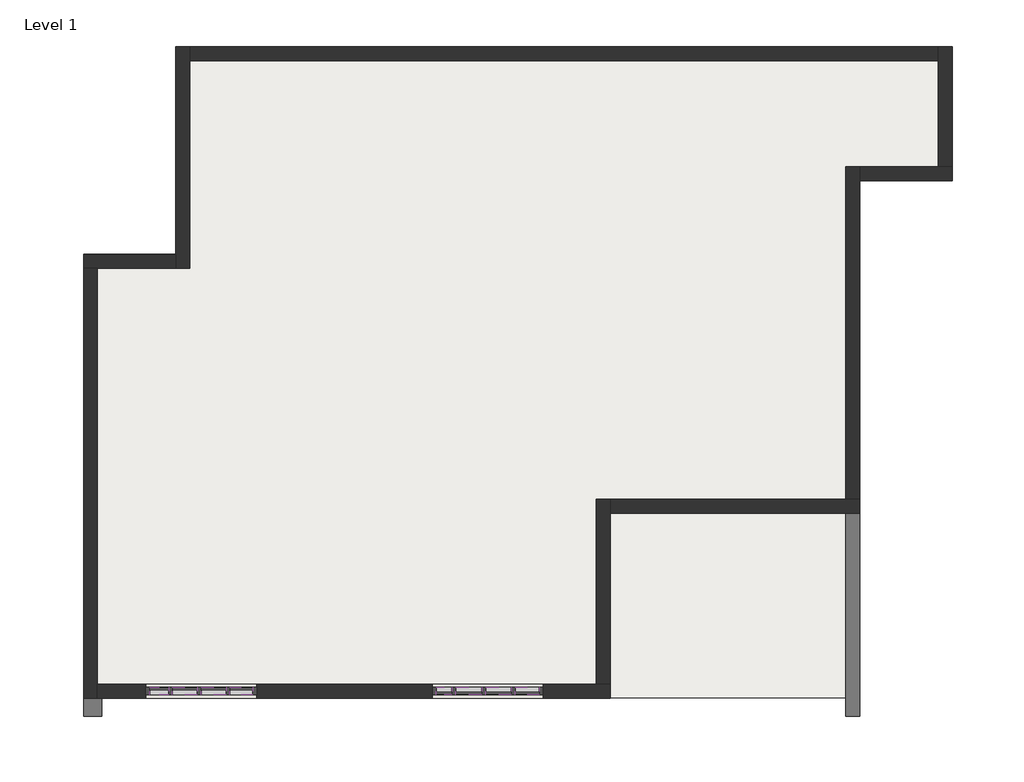
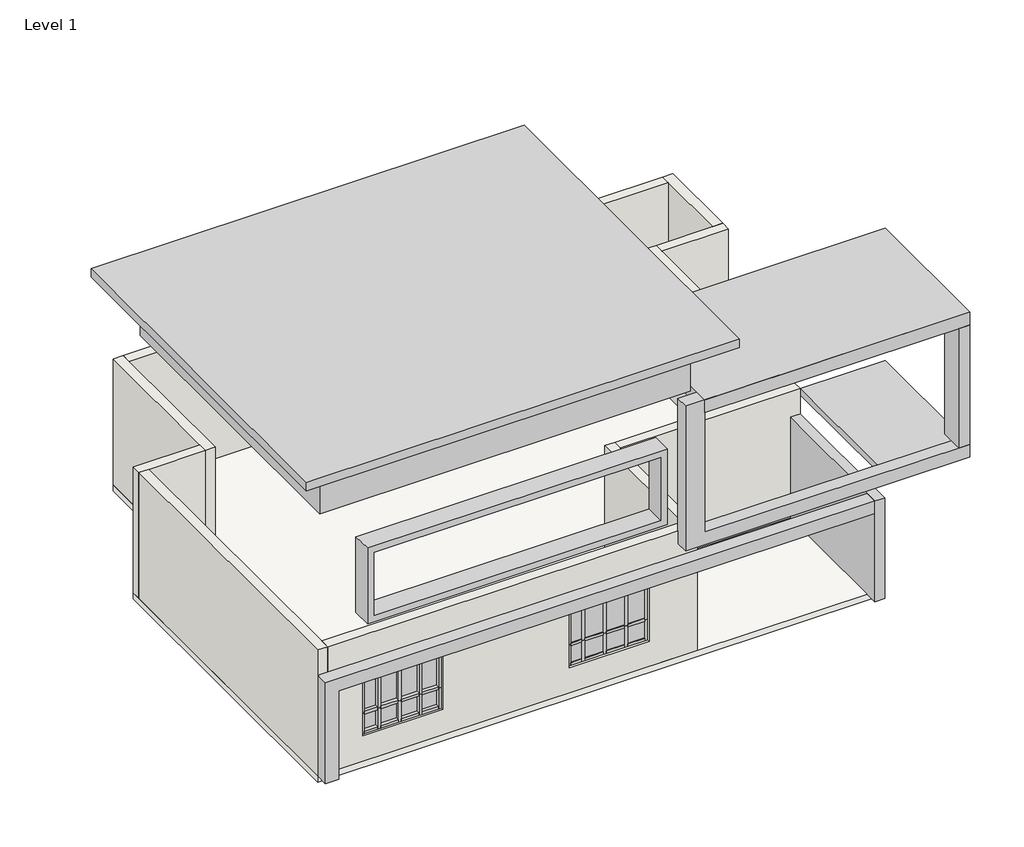
# One storey: 44 members, 16 plates, 10 walls, 1 proxy, 1 slab.
"""IFC4 building model written with IfcOpenShell, lengths in millimetres."""

from ifc_helpers import new_model, si_unit, frame, origin, origin_with_axes, place, context, project, spatial, polyline, outline, extrude, faceted_brep, transform, mapped, element, save
from components import generic_models_1_generic_models_1_da173db9, member_35330a42, member_5ad95953, member_90750a43, member_9850ab14, member_34d525fb, member_e756d367, member_8b1256c5, member_f92b8aa2, member_8e09d03a, member_7fd687a9, member_4adcbd6e, member_1c9dfce7, member_5ca2cede, member_be2dbdeb, member_cf238b44, member_39486dda, system_panel_glazed_bc497e33, system_panel_glazed_3f4378e1, system_panel_glazed_eeed78fb, system_panel_glazed_60bba13d, system_panel_glazed_ad989134, system_panel_glazed_d518dbe9, system_panel_glazed_4258910c, system_panel_glazed_d839e02d, system_panel_glazed_c56bea94, system_panel_glazed_323f7165, system_panel_glazed_9bb7629d, system_panel_glazed_ece2a562

model = new_model("IFC4")

# Units and contexts
model_context = context("Model", 3, world=origin())
ifc_project = project(units=[si_unit("LENGTHUNIT", "METRE", prefix="MILLI")], contexts=[model_context])

# Site, building, storey
site = spatial("IfcSite", under=ifc_project)
building = spatial("IfcBuilding", under=site)
storey = spatial("IfcBuildingStorey", under=building, Name="Level 1", Elevation=0.0)

# Proxy
placement = place(None, origin())
generic_models_1_generic_models_1_shape = generic_models_1_generic_models_1_da173db9(model_context)
element("IfcBuildingElementProxy", 1, Name="Generic Models 1 : Generic Models 1", ObjectType="Generic Models 1 : Generic Models 1", at=placement, inside=storey, context=model_context, shape_type="MappedRepresentation", body=[
    mapped(generic_models_1_generic_models_1_shape, transform((0.0, 0.0, 0.0), x_axis=(1.0, 0.0, 0.0), y_axis=(0.0, 1.0, 0.0), z_axis=(0.0, 0.0, 1.0))),
])

# Members
member_shape = member_35330a42(model_context)
element("IfcMember", 2, ObjectType="Rectangular Mullion : 2.5\" x 5\" rectangular", at=placement, inside=storey, context=model_context, shape_type="MappedRepresentation", body=[
    mapped(member_shape, transform((-4793.1680265, 1641.9286055, 2133.6), x_axis=(0.0, 0.0, 1.0), y_axis=(0.0, -1.0, 0.0), z_axis=(1.0, 0.0, 0.0))),
])
member_2_shape = member_5ad95953(model_context)
element("IfcMember", 3, ObjectType="Rectangular Mullion : 2.5\" x 5\" rectangular", at=placement, inside=storey, context=model_context, shape_type="MappedRepresentation", body=[
    mapped(member_2_shape, transform((-6494.9680265, 1641.9286055, 609.6), x_axis=(0.0, 0.0, -1.0), y_axis=(0.0, -1.0, 0.0), z_axis=(-1.0, 0.0, 0.0))),
])
member_3_shape = member_90750a43(model_context)
element("IfcMember", 4, ObjectType="Rectangular Mullion : 2.5\" x 5\" rectangular", at=placement, inside=storey, context=model_context, shape_type="MappedRepresentation", body=[
    mapped(member_3_shape, transform((-6152.0680265, 1641.9286055, 609.6), x_axis=(1.0, 0.0, 0.0), y_axis=(0.0, -1.0, 0.0), z_axis=(0.0, 0.0, -1.0))),
])
element("IfcMember", 5, ObjectType="Rectangular Mullion : 2.5\" x 5\" rectangular", at=placement, inside=storey, context=model_context, shape_type="MappedRepresentation", body=[
    mapped(member_3_shape, transform((-5677.9346932, 1641.9286055, 609.6), x_axis=(1.0, 0.0, 0.0), y_axis=(0.0, -1.0, 0.0), z_axis=(0.0, 0.0, -1.0))),
])
element("IfcMember", 6, ObjectType="Rectangular Mullion : 2.5\" x 5\" rectangular", at=placement, inside=storey, context=model_context, shape_type="MappedRepresentation", body=[
    mapped(member_3_shape, transform((-5203.8013599, 1641.9286055, 609.6), x_axis=(1.0, 0.0, 0.0), y_axis=(0.0, -1.0, 0.0), z_axis=(0.0, 0.0, -1.0))),
])
element("IfcMember", 7, ObjectType="Rectangular Mullion : 2.5\" x 5\" rectangular", at=placement, inside=storey, context=model_context, shape_type="MappedRepresentation", body=[
    mapped(member_3_shape, transform((-1478.4680265, 1641.9286055, 609.6), x_axis=(-1.0, 0.0, 0.0), y_axis=(0.0, 1.0, 0.0), z_axis=(0.0, 0.0, -1.0))),
])
element("IfcMember", 8, ObjectType="Rectangular Mullion : 2.5\" x 5\" rectangular", at=placement, inside=storey, context=model_context, shape_type="MappedRepresentation", body=[
    mapped(member_3_shape, transform((-987.4013599, 1641.9286055, 609.6), x_axis=(-1.0, 0.0, 0.0), y_axis=(0.0, 1.0, 0.0), z_axis=(0.0, 0.0, -1.0))),
])
element("IfcMember", 9, ObjectType="Rectangular Mullion : 2.5\" x 5\" rectangular", at=placement, inside=storey, context=model_context, shape_type="MappedRepresentation", body=[
    mapped(member_3_shape, transform((-496.3346932, 1641.9286055, 609.6), x_axis=(-1.0, 0.0, 0.0), y_axis=(0.0, 1.0, 0.0), z_axis=(0.0, 0.0, -1.0))),
])
member_4_shape = member_9850ab14(model_context)
element("IfcMember", 10, ObjectType="Rectangular Mullion : 2.5\" x 5\" rectangular", at=placement, inside=storey, context=model_context, shape_type="MappedRepresentation", body=[
    mapped(member_4_shape, transform((-6183.8180265, 1641.9286055, 1117.6), x_axis=(0.0, 0.0, 1.0), y_axis=(0.0, -1.0, 0.0), z_axis=(1.0, 0.0, 0.0))),
])
member_5_shape = member_34d525fb(model_context)
element("IfcMember", 11, ObjectType="Rectangular Mullion : 2.5\" x 5\" rectangular", at=placement, inside=storey, context=model_context, shape_type="MappedRepresentation", body=[
    mapped(member_5_shape, transform((-5709.6846932, 1641.9286055, 1117.6), x_axis=(0.0, 0.0, 1.0), y_axis=(0.0, -1.0, 0.0), z_axis=(1.0, 0.0, 0.0))),
])
element("IfcMember", 12, ObjectType="Rectangular Mullion : 2.5\" x 5\" rectangular", at=placement, inside=storey, context=model_context, shape_type="MappedRepresentation", body=[
    mapped(member_5_shape, transform((-5235.5513599, 1641.9286055, 1117.6), x_axis=(0.0, 0.0, 1.0), y_axis=(0.0, -1.0, 0.0), z_axis=(1.0, 0.0, 0.0))),
])
member_6_shape = member_e756d367(model_context)
element("IfcMember", 13, ObjectType="Rectangular Mullion : 2.5\" x 5\" rectangular", at=placement, inside=storey, context=model_context, shape_type="MappedRepresentation", body=[
    mapped(member_6_shape, transform((-4793.1680265, 1641.9286055, 1117.6), x_axis=(0.0, 0.0, 1.0), y_axis=(0.0, -1.0, 0.0), z_axis=(1.0, 0.0, 0.0))),
])
member_7_shape = member_8b1256c5(model_context)
element("IfcMember", 14, ObjectType="Rectangular Mullion : 2.5\" x 5\" rectangular", at=placement, inside=storey, context=model_context, shape_type="MappedRepresentation", body=[
    mapped(member_7_shape, transform((-6120.3180265, 1641.9286055, 609.6), x_axis=(0.0, 0.0, -1.0), y_axis=(0.0, -1.0, 0.0), z_axis=(-1.0, 0.0, 0.0))),
])
element("IfcMember", 15, ObjectType="Rectangular Mullion : 2.5\" x 5\" rectangular", at=placement, inside=storey, context=model_context, shape_type="MappedRepresentation", body=[
    mapped(member_7_shape, transform((-5646.1846932, 1641.9286055, 609.6), x_axis=(0.0, 0.0, -1.0), y_axis=(0.0, -1.0, 0.0), z_axis=(-1.0, 0.0, 0.0))),
])
element("IfcMember", 16, ObjectType="Rectangular Mullion : 2.5\" x 5\" rectangular", at=placement, inside=storey, context=model_context, shape_type="MappedRepresentation", body=[
    mapped(member_shape, transform((-5172.0513599, 1641.9286055, 609.6), x_axis=(0.0, 0.0, -1.0), y_axis=(0.0, -1.0, 0.0), z_axis=(-1.0, 0.0, 0.0))),
])
element("IfcMember", 17, ObjectType="Rectangular Mullion : 2.5\" x 5\" rectangular", at=placement, inside=storey, context=model_context, shape_type="MappedRepresentation", body=[
    mapped(member_2_shape, transform((-6183.8180265, 1641.9286055, 2133.6), x_axis=(0.0, 0.0, 1.0), y_axis=(0.0, -1.0, 0.0), z_axis=(1.0, 0.0, 0.0))),
])
element("IfcMember", 18, ObjectType="Rectangular Mullion : 2.5\" x 5\" rectangular", at=placement, inside=storey, context=model_context, shape_type="MappedRepresentation", body=[
    mapped(member_7_shape, transform((-5709.6846932, 1641.9286055, 2133.6), x_axis=(0.0, 0.0, 1.0), y_axis=(0.0, -1.0, 0.0), z_axis=(1.0, 0.0, 0.0))),
])
element("IfcMember", 19, ObjectType="Rectangular Mullion : 2.5\" x 5\" rectangular", at=placement, inside=storey, context=model_context, shape_type="MappedRepresentation", body=[
    mapped(member_7_shape, transform((-5235.5513599, 1641.9286055, 2133.6), x_axis=(0.0, 0.0, 1.0), y_axis=(0.0, -1.0, 0.0), z_axis=(1.0, 0.0, 0.0))),
])
member_8_shape = member_f92b8aa2(model_context)
element("IfcMember", 20, ObjectType="Rectangular Mullion : 2.5\" x 5\" rectangular", at=placement, inside=storey, context=model_context, shape_type="MappedRepresentation", body=[
    mapped(member_8_shape, transform((-6152.0680265, 1641.9286055, 1117.6), x_axis=(1.0, 0.0, 0.0), y_axis=(0.0, -1.0, 0.0), z_axis=(0.0, 0.0, -1.0))),
])
element("IfcMember", 21, ObjectType="Rectangular Mullion : 2.5\" x 5\" rectangular", at=placement, inside=storey, context=model_context, shape_type="MappedRepresentation", body=[
    mapped(member_8_shape, transform((-5677.9346932, 1641.9286055, 1117.6), x_axis=(1.0, 0.0, 0.0), y_axis=(0.0, -1.0, 0.0), z_axis=(0.0, 0.0, -1.0))),
])
element("IfcMember", 22, ObjectType="Rectangular Mullion : 2.5\" x 5\" rectangular", at=placement, inside=storey, context=model_context, shape_type="MappedRepresentation", body=[
    mapped(member_8_shape, transform((-5203.8013599, 1641.9286055, 1117.6), x_axis=(1.0, 0.0, 0.0), y_axis=(0.0, -1.0, 0.0), z_axis=(0.0, 0.0, -1.0))),
])
element("IfcMember", 23, ObjectType="Rectangular Mullion : 2.5\" x 5\" rectangular", at=placement, inside=storey, context=model_context, shape_type="MappedRepresentation", body=[
    mapped(member_8_shape, transform((-1478.4680265, 1641.9286055, 1117.6), x_axis=(-1.0, 0.0, 0.0), y_axis=(0.0, 1.0, 0.0), z_axis=(0.0, 0.0, -1.0))),
])
element("IfcMember", 24, ObjectType="Rectangular Mullion : 2.5\" x 5\" rectangular", at=placement, inside=storey, context=model_context, shape_type="MappedRepresentation", body=[
    mapped(member_8_shape, transform((-987.4013599, 1641.9286055, 1117.6), x_axis=(-1.0, 0.0, 0.0), y_axis=(0.0, 1.0, 0.0), z_axis=(0.0, 0.0, -1.0))),
])
element("IfcMember", 25, ObjectType="Rectangular Mullion : 2.5\" x 5\" rectangular", at=placement, inside=storey, context=model_context, shape_type="MappedRepresentation", body=[
    mapped(member_8_shape, transform((-496.3346932, 1641.9286055, 1117.6), x_axis=(-1.0, 0.0, 0.0), y_axis=(0.0, 1.0, 0.0), z_axis=(0.0, 0.0, -1.0))),
])
member_9_shape = member_8e09d03a(model_context)
element("IfcMember", 26, ObjectType="Rectangular Mullion : 2.5\" x 5\" rectangular", at=placement, inside=storey, context=model_context, shape_type="MappedRepresentation", body=[
    mapped(member_9_shape, transform((-6558.4680265, 1641.9286055, 2133.6), x_axis=(-1.0, 0.0, 0.0), y_axis=(0.0, -1.0, 0.0), z_axis=(0.0, 0.0, 1.0))),
])
element("IfcMember", 27, ObjectType="Rectangular Mullion : 2.5\" x 5\" rectangular", at=placement, inside=storey, context=model_context, shape_type="MappedRepresentation", body=[
    mapped(member_9_shape, transform((-5.2680265, 1641.9286055, 2133.6), x_axis=(1.0, 0.0, 0.0), y_axis=(0.0, 1.0, 0.0), z_axis=(0.0, 0.0, 1.0))),
])
member_10_shape = member_7fd687a9(model_context)
element("IfcMember", 28, ObjectType="Rectangular Mullion : 2.5\" x 5\" rectangular", at=placement, inside=storey, context=model_context, shape_type="MappedRepresentation", body=[
    mapped(member_10_shape, transform((-4729.6680265, 1641.9286055, 609.6), x_axis=(1.0, 0.0, 0.0), y_axis=(0.0, -1.0, 0.0), z_axis=(0.0, 0.0, -1.0))),
])
element("IfcMember", 29, ObjectType="Rectangular Mullion : 2.5\" x 5\" rectangular", at=placement, inside=storey, context=model_context, shape_type="MappedRepresentation", body=[
    mapped(member_10_shape, transform((-1834.0680265, 1641.9286055, 609.6), x_axis=(-1.0, 0.0, 0.0), y_axis=(0.0, 1.0, 0.0), z_axis=(0.0, 0.0, -1.0))),
])
element("IfcMember", 30, ObjectType="Rectangular Mullion : 2.5\" x 5\" rectangular", at=placement, inside=storey, context=model_context, shape_type="MappedRepresentation", body=[
    mapped(member_9_shape, transform((-4729.6680265, 1641.9286055, 1117.6), x_axis=(1.0, 0.0, 0.0), y_axis=(0.0, -1.0, 0.0), z_axis=(0.0, 0.0, -1.0))),
])
element("IfcMember", 31, ObjectType="Rectangular Mullion : 2.5\" x 5\" rectangular", at=placement, inside=storey, context=model_context, shape_type="MappedRepresentation", body=[
    mapped(member_9_shape, transform((-1834.0680265, 1641.9286055, 1117.6), x_axis=(-1.0, 0.0, 0.0), y_axis=(0.0, 1.0, 0.0), z_axis=(0.0, 0.0, -1.0))),
])
element("IfcMember", 32, ObjectType="Rectangular Mullion : 2.5\" x 5\" rectangular", at=placement, inside=storey, context=model_context, shape_type="MappedRepresentation", body=[
    mapped(member_10_shape, transform((-6558.4680265, 1641.9286055, 1117.6), x_axis=(-1.0, 0.0, 0.0), y_axis=(0.0, -1.0, 0.0), z_axis=(0.0, 0.0, 1.0))),
])
element("IfcMember", 33, ObjectType="Rectangular Mullion : 2.5\" x 5\" rectangular", at=placement, inside=storey, context=model_context, shape_type="MappedRepresentation", body=[
    mapped(member_10_shape, transform((-5.2680265, 1641.9286055, 1117.6), x_axis=(1.0, 0.0, 0.0), y_axis=(0.0, 1.0, 0.0), z_axis=(0.0, 0.0, 1.0))),
])
member_11_shape = member_4adcbd6e(model_context)
element("IfcMember", 34, ObjectType="Rectangular Mullion : 2.5\" x 5\" rectangular", at=placement, inside=storey, context=model_context, shape_type="MappedRepresentation", body=[
    mapped(member_11_shape, transform((-1770.5680265, 1641.9286055, 2133.6), x_axis=(0.0, 0.0, 1.0), y_axis=(0.0, 1.0, 0.0), z_axis=(-1.0, 0.0, 0.0))),
])
member_12_shape = member_1c9dfce7(model_context)
element("IfcMember", 35, ObjectType="Rectangular Mullion : 2.5\" x 5\" rectangular", at=placement, inside=storey, context=model_context, shape_type="MappedRepresentation", body=[
    mapped(member_12_shape, transform((-68.7680265, 1641.9286055, 609.6), x_axis=(0.0, 0.0, -1.0), y_axis=(0.0, 1.0, 0.0), z_axis=(1.0, 0.0, 0.0))),
])
member_13_shape = member_5ca2cede(model_context)
element("IfcMember", 36, ObjectType="Rectangular Mullion : 2.5\" x 5\" rectangular", at=placement, inside=storey, context=model_context, shape_type="MappedRepresentation", body=[
    mapped(member_13_shape, transform((-464.5846932, 1641.9286055, 1117.6), x_axis=(0.0, 0.0, 1.0), y_axis=(0.0, 1.0, 0.0), z_axis=(-1.0, 0.0, 0.0))),
])
member_14_shape = member_be2dbdeb(model_context)
element("IfcMember", 37, ObjectType="Rectangular Mullion : 2.5\" x 5\" rectangular", at=placement, inside=storey, context=model_context, shape_type="MappedRepresentation", body=[
    mapped(member_14_shape, transform((-1770.5680265, 1641.9286055, 1117.6), x_axis=(0.0, 0.0, 1.0), y_axis=(0.0, 1.0, 0.0), z_axis=(-1.0, 0.0, 0.0))),
])
member_15_shape = member_cf238b44(model_context)
element("IfcMember", 38, ObjectType="Rectangular Mullion : 2.5\" x 5\" rectangular", at=placement, inside=storey, context=model_context, shape_type="MappedRepresentation", body=[
    mapped(member_15_shape, transform((-1446.7180265, 1641.9286055, 1117.6), x_axis=(0.0, 0.0, 1.0), y_axis=(0.0, 1.0, 0.0), z_axis=(-1.0, 0.0, 0.0))),
])
element("IfcMember", 39, ObjectType="Rectangular Mullion : 2.5\" x 5\" rectangular", at=placement, inside=storey, context=model_context, shape_type="MappedRepresentation", body=[
    mapped(member_15_shape, transform((-955.6513599, 1641.9286055, 1117.6), x_axis=(0.0, 0.0, 1.0), y_axis=(0.0, 1.0, 0.0), z_axis=(-1.0, 0.0, 0.0))),
])
element("IfcMember", 40, ObjectType="Rectangular Mullion : 2.5\" x 5\" rectangular", at=placement, inside=storey, context=model_context, shape_type="MappedRepresentation", body=[
    mapped(member_11_shape, transform((-1510.2180265, 1641.9286055, 609.6), x_axis=(0.0, 0.0, -1.0), y_axis=(0.0, 1.0, 0.0), z_axis=(1.0, 0.0, 0.0))),
])
member_16_shape = member_39486dda(model_context)
element("IfcMember", 41, ObjectType="Rectangular Mullion : 2.5\" x 5\" rectangular", at=placement, inside=storey, context=model_context, shape_type="MappedRepresentation", body=[
    mapped(member_16_shape, transform((-1019.1513599, 1641.9286055, 609.6), x_axis=(0.0, 0.0, -1.0), y_axis=(0.0, 1.0, 0.0), z_axis=(1.0, 0.0, 0.0))),
])
element("IfcMember", 42, ObjectType="Rectangular Mullion : 2.5\" x 5\" rectangular", at=placement, inside=storey, context=model_context, shape_type="MappedRepresentation", body=[
    mapped(member_16_shape, transform((-528.0846932, 1641.9286055, 609.6), x_axis=(0.0, 0.0, -1.0), y_axis=(0.0, 1.0, 0.0), z_axis=(1.0, 0.0, 0.0))),
])
element("IfcMember", 43, ObjectType="Rectangular Mullion : 2.5\" x 5\" rectangular", at=placement, inside=storey, context=model_context, shape_type="MappedRepresentation", body=[
    mapped(member_16_shape, transform((-1446.7180265, 1641.9286055, 2133.6), x_axis=(0.0, 0.0, 1.0), y_axis=(0.0, 1.0, 0.0), z_axis=(-1.0, 0.0, 0.0))),
])
element("IfcMember", 44, ObjectType="Rectangular Mullion : 2.5\" x 5\" rectangular", at=placement, inside=storey, context=model_context, shape_type="MappedRepresentation", body=[
    mapped(member_16_shape, transform((-955.6513599, 1641.9286055, 2133.6), x_axis=(0.0, 0.0, 1.0), y_axis=(0.0, 1.0, 0.0), z_axis=(-1.0, 0.0, 0.0))),
])
element("IfcMember", 45, ObjectType="Rectangular Mullion : 2.5\" x 5\" rectangular", at=placement, inside=storey, context=model_context, shape_type="MappedRepresentation", body=[
    mapped(member_12_shape, transform((-464.5846932, 1641.9286055, 2133.6), x_axis=(0.0, 0.0, 1.0), y_axis=(0.0, 1.0, 0.0), z_axis=(-1.0, 0.0, 0.0))),
])

# Plates
system_panel_glazed_shape = system_panel_glazed_bc497e33(model_context)
element("IfcPlate", 46, ObjectType="System Panel : Glazed", at=placement, inside=storey, context=model_context, shape_type="MappedRepresentation", body=[
    mapped(system_panel_glazed_shape, transform((-6339.3930265, 1641.9286055, 673.1), x_axis=(1.0, 0.0, 0.0), y_axis=(0.0, 1.0, 0.0), z_axis=(0.0, 0.0, 1.0))),
])
system_panel_glazed_2_shape = system_panel_glazed_3f4378e1(model_context)
element("IfcPlate", 47, ObjectType="System Panel : Glazed", at=placement, inside=storey, context=model_context, shape_type="MappedRepresentation", body=[
    mapped(system_panel_glazed_2_shape, transform((-5915.0013599, 1641.9286055, 673.1), x_axis=(1.0, 0.0, 0.0), y_axis=(0.0, 1.0, 0.0), z_axis=(0.0, 0.0, 1.0))),
])
element("IfcPlate", 48, ObjectType="System Panel : Glazed", at=placement, inside=storey, context=model_context, shape_type="MappedRepresentation", body=[
    mapped(system_panel_glazed_2_shape, transform((-5440.8680265, 1641.9286055, 673.1), x_axis=(1.0, 0.0, 0.0), y_axis=(0.0, 1.0, 0.0), z_axis=(0.0, 0.0, 1.0))),
])
system_panel_glazed_3_shape = system_panel_glazed_eeed78fb(model_context)
element("IfcPlate", 49, ObjectType="System Panel : Glazed", at=placement, inside=storey, context=model_context, shape_type="MappedRepresentation", body=[
    mapped(system_panel_glazed_3_shape, transform((-4982.6096932, 1641.9286055, 673.1), x_axis=(1.0, 0.0, 0.0), y_axis=(0.0, 1.0, 0.0), z_axis=(0.0, 0.0, 1.0))),
])
system_panel_glazed_4_shape = system_panel_glazed_60bba13d(model_context)
element("IfcPlate", 50, ObjectType="System Panel : Glazed", at=placement, inside=storey, context=model_context, shape_type="MappedRepresentation", body=[
    mapped(system_panel_glazed_4_shape, transform((-6339.3930265, 1641.9286055, 1149.35), x_axis=(1.0, 0.0, 0.0), y_axis=(0.0, 1.0, 0.0), z_axis=(0.0, 0.0, 1.0))),
])
system_panel_glazed_5_shape = system_panel_glazed_ad989134(model_context)
element("IfcPlate", 51, ObjectType="System Panel : Glazed", at=placement, inside=storey, context=model_context, shape_type="MappedRepresentation", body=[
    mapped(system_panel_glazed_5_shape, transform((-5915.0013599, 1641.9286055, 1149.35), x_axis=(1.0, 0.0, 0.0), y_axis=(0.0, 1.0, 0.0), z_axis=(0.0, 0.0, 1.0))),
])
element("IfcPlate", 52, ObjectType="System Panel : Glazed", at=placement, inside=storey, context=model_context, shape_type="MappedRepresentation", body=[
    mapped(system_panel_glazed_5_shape, transform((-5440.8680265, 1641.9286055, 1149.35), x_axis=(1.0, 0.0, 0.0), y_axis=(0.0, 1.0, 0.0), z_axis=(0.0, 0.0, 1.0))),
])
system_panel_glazed_6_shape = system_panel_glazed_d518dbe9(model_context)
element("IfcPlate", 53, ObjectType="System Panel : Glazed", at=placement, inside=storey, context=model_context, shape_type="MappedRepresentation", body=[
    mapped(system_panel_glazed_6_shape, transform((-4982.6096932, 1641.9286055, 1149.35), x_axis=(1.0, 0.0, 0.0), y_axis=(0.0, 1.0, 0.0), z_axis=(0.0, 0.0, 1.0))),
])
system_panel_glazed_7_shape = system_panel_glazed_4258910c(model_context)
element("IfcPlate", 54, ObjectType="System Panel : Glazed", at=placement, inside=storey, context=model_context, shape_type="MappedRepresentation", body=[
    mapped(system_panel_glazed_7_shape, transform((-266.6763599, 1641.9286055, 673.1), x_axis=(-1.0, 0.0, 0.0), y_axis=(0.0, -1.0, 0.0), z_axis=(0.0, 0.0, 1.0))),
])
system_panel_glazed_8_shape = system_panel_glazed_d839e02d(model_context)
element("IfcPlate", 55, ObjectType="System Panel : Glazed", at=placement, inside=storey, context=model_context, shape_type="MappedRepresentation", body=[
    mapped(system_panel_glazed_8_shape, transform((-1640.3930265, 1641.9286055, 673.1), x_axis=(-1.0, 0.0, 0.0), y_axis=(0.0, -1.0, 0.0), z_axis=(0.0, 0.0, 1.0))),
])
system_panel_glazed_9_shape = system_panel_glazed_c56bea94(model_context)
element("IfcPlate", 56, ObjectType="System Panel : Glazed", at=placement, inside=storey, context=model_context, shape_type="MappedRepresentation", body=[
    mapped(system_panel_glazed_9_shape, transform((-1232.9346932, 1641.9286055, 673.1), x_axis=(-1.0, 0.0, 0.0), y_axis=(0.0, -1.0, 0.0), z_axis=(0.0, 0.0, 1.0))),
])
element("IfcPlate", 57, ObjectType="System Panel : Glazed", at=placement, inside=storey, context=model_context, shape_type="MappedRepresentation", body=[
    mapped(system_panel_glazed_9_shape, transform((-741.8680265, 1641.9286055, 673.1), x_axis=(-1.0, 0.0, 0.0), y_axis=(0.0, -1.0, 0.0), z_axis=(0.0, 0.0, 1.0))),
])
system_panel_glazed_10_shape = system_panel_glazed_323f7165(model_context)
element("IfcPlate", 58, ObjectType="System Panel : Glazed", at=placement, inside=storey, context=model_context, shape_type="MappedRepresentation", body=[
    mapped(system_panel_glazed_10_shape, transform((-266.6763599, 1641.9286055, 1149.35), x_axis=(-1.0, 0.0, 0.0), y_axis=(0.0, -1.0, 0.0), z_axis=(0.0, 0.0, 1.0))),
])
system_panel_glazed_11_shape = system_panel_glazed_9bb7629d(model_context)
element("IfcPlate", 59, ObjectType="System Panel : Glazed", at=placement, inside=storey, context=model_context, shape_type="MappedRepresentation", body=[
    mapped(system_panel_glazed_11_shape, transform((-741.8680265, 1641.9286055, 1149.35), x_axis=(-1.0, 0.0, 0.0), y_axis=(0.0, -1.0, 0.0), z_axis=(0.0, 0.0, 1.0))),
])
element("IfcPlate", 60, ObjectType="System Panel : Glazed", at=placement, inside=storey, context=model_context, shape_type="MappedRepresentation", body=[
    mapped(system_panel_glazed_11_shape, transform((-1232.9346932, 1641.9286055, 1149.35), x_axis=(-1.0, 0.0, 0.0), y_axis=(0.0, -1.0, 0.0), z_axis=(0.0, 0.0, 1.0))),
])
system_panel_glazed_12_shape = system_panel_glazed_ece2a562(model_context)
element("IfcPlate", 61, ObjectType="System Panel : Glazed", at=placement, inside=storey, context=model_context, shape_type="MappedRepresentation", body=[
    mapped(system_panel_glazed_12_shape, transform((-1640.3930265, 1641.9286055, 1149.35), x_axis=(-1.0, 0.0, 0.0), y_axis=(0.0, -1.0, 0.0), z_axis=(0.0, 0.0, 1.0))),
])

# Slab
element("IfcSlab", 62, ObjectType="6\"", at=placement, inside=storey, context=model_context, shape_type="SweptSolid", body=[
    extrude(outline(polyline([(-6063.1680265, 12273.6040735), (6738.4319735, 12273.6040735), (6738.4319735, 10063.8040735), (5214.4319735, 10063.8040735), (5214.4319735, 1529.4040735), (-7587.1680265, 1529.4040735), (-7587.1680265, 8844.6040735), (-6063.1680265, 8844.6040735), (-6063.1680265, 12273.6040735)])), frame((0.0, 0.0, -152.4206871), z_axis=(0.0, 0.0, 1.0), x_axis=(1.0, 0.0, 0.0)), (0.0, 0.0, 1.0), 152.4),
])

# Walls
element("IfcWall", 63, ObjectType="9\" wall", at=placement, inside=storey, context=model_context, shape_type="Brep", body=[
    faceted_brep([(-6063.1680265, 12271.8286055, 0.0), (-6063.1680265, 8842.8286055, 0.0), (-6063.1680265, 8614.2286055, 0.0), (-6063.1680265, 8614.2286055, 3048.0), (-6063.1680265, 8842.8286055, 3048.0), (-6063.1680265, 12271.8286055, 3048.0), (-5834.5680265, 12271.8286055, 0.0), (-5834.5680265, 12271.8286055, 3048.0), (-5834.5680265, 12043.2286055, 3048.0), (-5834.5680265, 8614.2286055, 3048.0), (-5834.5680265, 8614.2286055, 0.0), (-5834.5680265, 12043.2286055, 0.0)], [[[0, 1, 2, 3, 4, 5]], [[6, 7, 8, 9, 10, 11]], [[2, 1, 0, 6, 11, 10]], [[5, 4, 3, 9, 8, 7]], [[3, 2, 10, 9]], [[0, 5, 7, 6]]]),
])
element("IfcWall", 64, ObjectType="9\" wall", at=placement, inside=storey, context=model_context, shape_type="Brep", body=[
    faceted_brep([(-6063.1680265, 8842.8286055, 0.0), (-7587.1680265, 8842.8286055, 0.0), (-7587.1680265, 8842.8286055, 3048.0), (-6063.1680265, 8842.8286055, 3048.0), (-6063.1680265, 8614.2286055, 0.0), (-6063.1680265, 8614.2286055, 3048.0), (-7358.5680265, 8614.2286055, 3048.0), (-7587.1680265, 8614.2286055, 3048.0), (-7587.1680265, 8614.2286055, 0.0), (-7358.5680265, 8614.2286055, 0.0)], [[[0, 1, 2, 3]], [[4, 5, 6, 7, 8, 9]], [[1, 0, 4, 9, 8]], [[3, 2, 7, 6, 5]], [[0, 3, 5, 4]], [[2, 1, 8, 7]]]),
])
element("IfcWall", 65, ObjectType="9\" wall", at=placement, inside=storey, context=model_context, shape_type="Brep", body=[
    faceted_brep([(-7587.1680265, 8614.2286055, 0.0), (-7587.1680265, 1527.6286055, 0.0), (-7587.1680265, 1527.6286055, 3048.0), (-7587.1680265, 8614.2286055, 3048.0), (-7358.5680265, 8614.2286055, 0.0), (-7358.5680265, 8614.2286055, 3048.0), (-7358.5680265, 1756.2286055, 3048.0), (-7358.5680265, 1527.6286055, 3048.0), (-7358.5680265, 1527.6286055, 0.0), (-7358.5680265, 1756.2286055, 0.0)], [[[0, 1, 2, 3]], [[4, 5, 6, 7, 8, 9]], [[1, 0, 4, 9, 8]], [[3, 2, 7, 6, 5]], [[0, 3, 5, 4]], [[2, 1, 8, 7]]]),
])
element("IfcWall", 66, ObjectType="9\" wall", at=placement, inside=storey, context=model_context, shape_type="Brep", body=[
    faceted_brep([(-7358.5680265, 1527.6286055, 0.0), (1099.6319735, 1527.6286055, 0.0), (1099.6319735, 1527.6286055, 3048.0), (-7358.5680265, 1527.6286055, 3048.0), (-6558.4680265, 1527.6286055, 609.6), (-6558.4680265, 1527.6286055, 2133.6), (-4729.6680265, 1527.6286055, 2133.6), (-4729.6680265, 1527.6286055, 609.6), (-5.2680265, 1527.6286055, 2133.6), (-5.2680265, 1527.6286055, 609.6), (-1834.0680265, 1527.6286055, 609.6), (-1834.0680265, 1527.6286055, 2133.6), (1099.6319735, 1756.2286055, 0.0), (871.0319735, 1756.2286055, 0.0), (-7358.5680265, 1756.2286055, 0.0), (-7358.5680265, 1756.2286055, 3048.0), (871.0319735, 1756.2286055, 3048.0), (1099.6319735, 1756.2286055, 3048.0), (-6558.4680265, 1756.2286055, 2133.6), (-6558.4680265, 1756.2286055, 609.6), (-4729.6680265, 1756.2286055, 609.6), (-4729.6680265, 1756.2286055, 2133.6), (-5.2680265, 1756.2286055, 609.6), (-5.2680265, 1756.2286055, 2133.6), (-1834.0680265, 1756.2286055, 2133.6), (-1834.0680265, 1756.2286055, 609.6)], [[[0, 1, 2, 3], [4, 5, 6, 7], [8, 9, 10, 11]], [[12, 13, 14, 15, 16, 17], [18, 19, 20, 21], [22, 23, 24, 25]], [[1, 0, 14, 13, 12]], [[3, 2, 17, 16, 15]], [[0, 3, 15, 14]], [[2, 1, 12, 17]], [[4, 19, 18, 5]], [[5, 18, 21, 6]], [[6, 21, 20, 7]], [[19, 4, 7, 20]], [[22, 9, 8, 23]], [[23, 8, 11, 24]], [[10, 25, 24, 11]], [[9, 22, 25, 10]]]),
])
element("IfcWall", 67, ObjectType="9\" wall", at=placement, inside=storey, context=model_context, shape_type="Brep", body=[
    faceted_brep([(1099.6319735, 1756.2286055, 0.0), (1099.6319735, 4575.6286055, 0.0), (1099.6319735, 4804.2286055, 0.0), (1099.6319735, 4804.2286055, 3048.0), (1099.6319735, 4575.6286055, 3048.0), (1099.6319735, 1756.2286055, 3048.0), (871.0319735, 1756.2286055, 0.0), (871.0319735, 1756.2286055, 3048.0), (871.0319735, 4804.2286055, 3048.0), (871.0319735, 4804.2286055, 0.0)], [[[0, 1, 2, 3, 4, 5]], [[6, 7, 8, 9]], [[2, 1, 0, 6, 9]], [[5, 4, 3, 8, 7]], [[0, 5, 7, 6]], [[3, 2, 9, 8]]]),
])
element("IfcWall", 68, ObjectType="9\" wall", at=placement, inside=storey, context=model_context, shape_type="Brep", body=[
    faceted_brep([(1099.6319735, 4575.6286055, 0.0), (5214.4319735, 4575.6286055, 0.0), (5214.4319735, 4575.6286055, 3048.0), (1099.6319735, 4575.6286055, 3048.0), (1099.6319735, 4804.2286055, 0.0), (1099.6319735, 4804.2286055, 3048.0), (4985.8319735, 4804.2286055, 3048.0), (5214.4319735, 4804.2286055, 3048.0), (5214.4319735, 4804.2286055, 0.0), (4985.8319735, 4804.2286055, 0.0)], [[[0, 1, 2, 3]], [[4, 5, 6, 7, 8, 9]], [[1, 0, 4, 9, 8]], [[3, 2, 7, 6, 5]], [[0, 3, 5, 4]], [[2, 1, 8, 7]]]),
])
element("IfcWall", 69, ObjectType="9\" wall", at=placement, inside=storey, context=model_context, shape_type="Brep", body=[
    faceted_brep([(5214.4319735, 4804.2286055, 0.0), (5214.4319735, 10062.0286055, 0.0), (5214.4319735, 10290.6286055, 0.0), (5214.4319735, 10290.6286055, 3048.0), (5214.4319735, 10062.0286055, 3048.0), (5214.4319735, 4804.2286055, 3048.0), (4985.8319735, 4804.2286055, 0.0), (4985.8319735, 4804.2286055, 3048.0), (4985.8319735, 10290.6286055, 3048.0), (4985.8319735, 10290.6286055, 0.0)], [[[0, 1, 2, 3, 4, 5]], [[6, 7, 8, 9]], [[2, 1, 0, 6, 9]], [[5, 4, 3, 8, 7]], [[0, 5, 7, 6]], [[3, 2, 9, 8]]]),
])
element("IfcWall", 70, ObjectType="9\" wall", at=placement, inside=storey, context=model_context, shape_type="Brep", body=[
    faceted_brep([(5214.4319735, 10062.0286055, 0.0), (6738.4319735, 10062.0286055, 0.0), (6738.4319735, 10062.0286055, 3048.0), (5214.4319735, 10062.0286055, 3048.0), (5214.4319735, 10290.6286055, 0.0), (5214.4319735, 10290.6286055, 3048.0), (6509.8319735, 10290.6286055, 3048.0), (6738.4319735, 10290.6286055, 3048.0), (6738.4319735, 10290.6286055, 0.0), (6509.8319735, 10290.6286055, 0.0)], [[[0, 1, 2, 3]], [[4, 5, 6, 7, 8, 9]], [[1, 0, 4, 9, 8]], [[3, 2, 7, 6, 5]], [[0, 3, 5, 4]], [[2, 1, 8, 7]]]),
])
element("IfcWall", 71, ObjectType="9\" wall", at=placement, inside=storey, context=model_context, shape_type="Brep", body=[
    faceted_brep([(6738.4319735, 10290.6286055, 0.0), (6738.4319735, 12271.8286055, 0.0), (6738.4319735, 12271.8286055, 3048.0), (6738.4319735, 10290.6286055, 3048.0), (6509.8319735, 10290.6286055, 0.0), (6509.8319735, 10290.6286055, 3048.0), (6509.8319735, 12043.2286055, 3048.0), (6509.8319735, 12271.8286055, 3048.0), (6509.8319735, 12271.8286055, 0.0), (6509.8319735, 12043.2286055, 0.0)], [[[0, 1, 2, 3]], [[4, 5, 6, 7, 8, 9]], [[1, 0, 4, 9, 8]], [[3, 2, 7, 6, 5]], [[0, 3, 5, 4]], [[2, 1, 8, 7]]]),
])
element("IfcWall", 72, ObjectType="9\" wall", at=placement, inside=storey, context=model_context, shape_type="SweptSolid", body=[
    extrude(outline(polyline([(-5834.5680265, 12271.8286055), (6509.8319735, 12271.8286055), (6509.8319735, 12043.2286055), (-5834.5680265, 12043.2286055), (-5834.5680265, 12271.8286055)])), origin_with_axes(), (0.0, 0.0, 1.0), 3048.0),
])

save(model, "model.ifc")

# Revit data of these elements
# Type "Rectangular Mullion : 2.5\" x 5\" rectangular"
#   built-in parameter 1007304 = 0.416667 (stored number, unit not read)
#   built-in parameter 1007301 = 0.104167 (stored number, unit not read)
#   built-in parameter 1007300 = 0.104167 (stored number, unit not read)
# Type "System Panel : Glazed"
#   Construction Type Id = "GSP4R"
#   Analytic Construction = "1/8 in Pilkington single glazing"
#   Visual Light Transmittance = 0.9
#   Solar Heat Gain Coefficient = 0.86
#   Heat Transfer Coefficient (U) = 1.18115 BTU/(h·ft²·°F)
#   Define Thermal Properties by = 1
# Type "6\""
#   Assembly Code = "B1010"
#   Function = 0
#   Layers, outside or top first: 0' - 6" "Gypsum Wall Board" (function 1)
# Type "9\" wall"
#   Assembly Code = "B2010"
#   Layers, outside or top first: 0' - 9" "Gypsum Wall Board" (function 1)
# Element 1 (IfcBuildingElementProxy, "Generic Models 1 : Generic Models 1")
#   Phase Created = New Construction
#   Materials on its faces: "Gypsum Wall Board", "extrusion", "tile"
# Elements 2, 3, 4, 5, 6, 7, 8, 9, 10, 11, 12, 13, 14, 15, 16, 17, 18, 19, 20, 21, 22, 23, 24, 25, 26, 27, 28, 29, 30, 31, 32, 33, 34, 35, 36, 37, 38, 39, 40, 41, 42, 43, 44, 45 (IfcMember, "Rectangular Mullion : 2.5\" x 5\" rectangular")
#   Phase Created = New Construction
# Elements 46, 47, 48, 49, 50, 51, 52, 53, 54, 55, 56, 57, 58, 59, 60, 61 (IfcPlate, "System Panel : Glazed")
#   Phase Created = New Construction
#   Materials on its faces: "Glass"
# Element 62 (IfcSlab, "6\"")
#   built-in parameter 1001955 = 3.14159 (stored number, unit not read)
#   Height Offset From Level = -0' - 0.00081"
#   Phase Created = New Construction
#   Materials on its faces: "Gypsum Wall Board"
# Elements 63, 64, 65, 66, 67, 68, 69, 70, 71, 72 (IfcWall, "9\" wall")
#   Top Offset = 0' - 0"
#   Base Offset = 0' - 0"
#   wall height = 10' - 0"
#   Phase Created = New Construction
#   Base Constraint = Level 1
#   Top Constraint = Level 2
#   Materials on its faces: "Gypsum Wall Board"
# Materials
#   "Gypsum Wall Board": class "Generic", colour RGB 127 127 127, transparency 0, Description = "Gypsum Wall Board", Cost = 0
#   "extrusion": class "Generic", colour RGB 120 120 120, transparency 0, Cost = 0
#   "tile": class "Generic", colour RGB 120 120 120, transparency 0, Cost = 0
#   "Glass": class "Glass", colour RGB 0 128 192, transparency 0.75, Description = "Soda Lime Glass", Cost = 0
